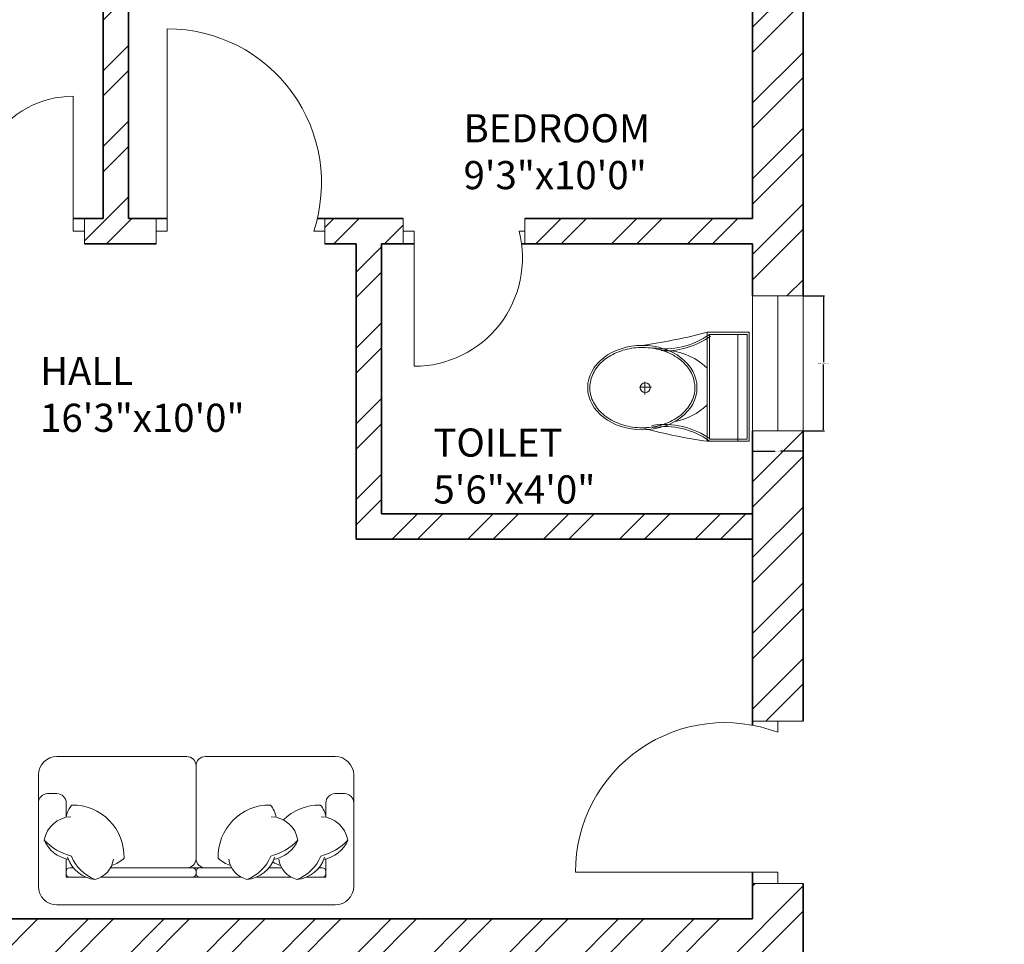
# Model space of a CAD drawing. Units: inches. Extents: x 2552 to 3217, y 1417 to 2737.
# Tile 10 of 25: x 2710 to 2885, y 2138 to 2302. Entities that reach past the tile are written whole.
import ezdxf

# ---------------------------------------------------------------- set-up
doc = ezdxf.new("R2010")
doc.units = ezdxf.units.IN
for name, color, linetype, lineweight in [('A-ANNO-DIMS', 2, 'Continuous', 18), ('A-AREA-IDEN', 7, 'Continuous', 18), ('A-DOOR', 21, 'Continuous', 18), ('A-FLOR-FIXT', 8, 'Continuous', 18), ('A-FURN', 8, 'Continuous', 13), ('A-GLAZ', 161, 'Continuous', 18), ('A-WALL', 7, 'Continuous', 35), ('A-WALL-PATT', 217, 'Continuous', 13)]:
    doc.layers.add(name, color=color, linetype=linetype, lineweight=lineweight)
doc.styles.get("Standard").update_dxf_attribs({"font": 'arial.ttf'})
doc.dimstyles.get("Standard").update_dxf_attribs({"dimtxt": 0.18, "dimasz": 0.18, "dimexe": 0.18, "dimexo": 0.0625, "dimgap": 0.09, "dimtad": 0, "dimtih": 1, "dimtoh": 1, "dimdec": 4, "dimzin": 0, "dimdsep": 46, "dimtxsty": 'Standard', "dimcen": 0.09, "dimadec": 0, "dimazin": 0, "dimtfac": 1, "dimtdec": 4, "dimtofl": 0, "dimtmove": 0, "dimatfit": 3, "dimfxl": 1, "dimtolj": 1, "dimtzin": 0, "dimarcsym": 0})

# ---------------------------------------------------------------- blocks, each defined once
blk = doc.blocks.new('A$C31115884')
for p, q in [((257.5, 466.4), (257.5, 523.2)), ((283.1, 497.7), (223.4, 497.7)), ((0, 200), (0, 0)), ((520, 200), (0, 200)), ((10, 190), (10, 10)), ((510, 190), (10, 190)), ((510, 10), (510, 190)), ((520, 0), (520, 200)), ((510, 54.5), (0, 54.5)), ((10, 10), (510, 10)), ((0, 0), (520, 0))]:
    blk.add_line(p, q)
blk.add_circle((255.6, 496.4), 23.6)
for centre, radius, start, end in [((2777.7, -204.6), 2807, 165.4549, 171.7133), ((3237, 905), 2807, 188.2867, 194.5451), ((-294.5, 403.3), 364.7, 324.2091, 9.3499), ((-294.5, 403.3), 374.7, 324.2091, 9.3499), ((805.8, 403.3), 364.7, 170.6501, 215.7909), ((139.5, 406.2), 293.5, 315.8436, 2.6563), ((805.8, 403.3), 374.7, 179.2036, 215.7909), ((383.6, 406.2), 293.5, 190.2774, 224.1564)]:
    blk.add_arc(centre, radius, start, end)
blk.add_ellipse((256.2, 509.9), major_axis=(0, -260.7), ratio=0.772727)
blk.add_open_spline([(256.2, 259.2), (263.1, 259.2), (270, 259.7), (287.8, 262.3), (298.7, 265.1), (319.9, 273.1), (330.2, 278.4), (350.1, 291.1), (359.7, 298.7), (377.7, 315.9), (386.2, 325.5), (401.7, 346.6), (408.8, 358.1), (421.3, 382.5), (426.8, 395.5), (435.9, 422.4), (439.5, 436.4), (444.8, 465.1), (446.5, 479.7), (447.9, 509.2), (447.6, 524), (445, 553.3), (442.7, 567.8), (436.3, 596), (432.1, 609.7), (421.9, 636), (416, 648.6), (402.5, 672.1), (395, 683), (378.6, 703), (369.8, 712.1), (351.1, 728), (341.3, 734.8), (320.9, 746.2), (310.4, 750.7), (288.9, 757.3), (278, 759.4), (256, 761), (245, 760.6), (223.1, 757.2), (212.3, 754.3), (191.1, 746.1), (180.8, 740.7), (160.9, 727.8), (151.4, 720.1), (133.5, 702.7), (125.1, 693), (109.6, 671.7), (102.6, 660.2), (90.2, 635.7), (84.9, 622.7), (76, 595.6), (72.4, 581.6), (67.2, 552.9), (65.6, 538.2), (64.4, 508.8), (64.8, 494), (67.5, 464.7), (69.9, 450.2), (76.6, 422), (80.8, 408.3), (91.1, 382.2), (97.2, 369.7), (110.8, 346.3), (118.4, 335.4), (134.8, 315.6), (143.7, 306.7), (162.4, 290.9), (172.3, 284.2), (192.8, 273), (203.3, 268.6), (224.8, 262.2), (235.8, 260.2), (249.9, 259.3), (253, 259.2), (256.2, 259.2)], degree=3, knots=[0, 0, 0, 0, 0.110105, 0.110105, 0.285049, 0.285049, 0.459994, 0.459994, 0.634938, 0.634938, 0.809882, 0.809882, 0.984827, 0.984827, 1.159771, 1.159771, 1.334715, 1.334715, 1.50966, 1.50966, 1.684604, 1.684604, 1.859549, 1.859549, 2.034493, 2.034493, 2.209437, 2.209437, 2.384382, 2.384382, 2.559326, 2.559326, 2.73427, 2.73427, 2.909215, 2.909215, 3.084159, 3.084159, 3.259103, 3.259103, 3.434048, 3.434048, 3.608992, 3.608992, 3.783936, 3.783936, 3.958881, 3.958881, 4.133825, 4.133825, 4.30877, 4.30877, 4.483714, 4.483714, 4.658658, 4.658658, 4.833603, 4.833603, 5.008547, 5.008547, 5.183491, 5.183491, 5.358436, 5.358436, 5.53338, 5.53338, 5.708324, 5.708324, 5.883269, 5.883269, 6.058213, 6.058213, 6.233158, 6.233158, 6.283185, 6.283185, 6.283185, 6.283185])
blk = doc.blocks.new('WIN-24')
for p, q in [((0, 24), (9, 24)), ((0, 24), (0, 0)), ((9, 24), (4.5, 24)), ((4.5, 24), (4.5, 0)), ((9, 24), (9, 0)), ((4.5, 0), (0, 0)), ((0, 0), (9, 0))]:
    blk.add_line(p, q)
blk = doc.blocks.new('*D25')
at = {"layer": 'A-ANNO-DIMS', "color": 0, "lineweight": -2, "transparency": 16777216}
for p, q in [((2848.92, 2253.28), (2852.63, 2253.28)), ((2852.45, 2253.1), (2852.45, 2241.47)), ((2852.45, 2229.46), (2852.45, 2241.1)), ((2848.92, 2229.28), (2852.63, 2229.28))]:
    blk.add_line(p, q, dxfattribs=at)
at = {"layer": 'A-ANNO-DIMS', "color": 0, "transparency": 16777216}
for points in [[(2852.42, 2253.1), (2852.48, 2253.1), (2852.45, 2253.28)], [(2852.42, 2229.46), (2852.48, 2229.46), (2852.45, 2229.28)]]:
    blk.add_solid(points, dxfattribs=at)
at = {"layer": 'Defpoints', "color": 0, "transparency": 16777216}
for p in [(2848.85, 2253.28), (2852.45, 2253.28), (2848.85, 2229.28)]:
    blk.add_point(p, dxfattribs=at)
at = {"layer": 'A-ANNO-DIMS', "color": 0, "transparency": 16777216, "insert": (2852.45, 2241.28), "char_height": 0.18, "attachment_point": 5}
blk.add_mtext('\\A1;WINDOW 24 TYP.', dxfattribs=at)
blk = doc.blocks.new('*D26')
at = {"layer": 'A-ANNO-DIMS', "color": 0, "lineweight": -2, "transparency": 16777216}
for p, q in [((2839.85, 2229.22), (2839.85, 2225.5)), ((2848.85, 2229.22), (2848.85, 2225.5)), ((2840.03, 2225.68), (2843.9, 2225.68)), ((2848.67, 2225.68), (2844.81, 2225.68))]:
    blk.add_line(p, q, dxfattribs=at)
at = {"layer": 'A-ANNO-DIMS', "color": 0, "transparency": 16777216}
for points in [[(2840.03, 2225.71), (2840.03, 2225.65), (2839.85, 2225.68)], [(2848.67, 2225.71), (2848.67, 2225.65), (2848.85, 2225.68)]]:
    blk.add_solid(points, dxfattribs=at)
at = {"layer": 'Defpoints', "color": 0, "transparency": 16777216}
for p in [(2839.85, 2229.28), (2848.85, 2229.28), (2848.85, 2225.68)]:
    blk.add_point(p, dxfattribs=at)
at = {"layer": 'A-ANNO-DIMS', "color": 0, "transparency": 16777216, "insert": (2844.35, 2225.68), "char_height": 0.18, "attachment_point": 5}
blk.add_mtext('\\A1;9 TYP.', dxfattribs=at)
blk = doc.blocks.new('*D64')
at = {"layer": 'A-ANNO-DIMS', "color": 0, "lineweight": -2, "transparency": 16777216}
for p, q in [((2646.35, 1551.58), (2646.35, 2709.49)), ((2646.53, 2709.31), (2802.77, 2709.31)), ((2959.93, 2709.31), (2803.69, 2709.31)), ((2960.11, 1551.58), (2960.11, 2709.49))]:
    blk.add_line(p, q, dxfattribs=at)
at = {"layer": 'A-ANNO-DIMS', "color": 0, "transparency": 16777216}
for points in [[(2646.53, 2709.34), (2646.53, 2709.28), (2646.35, 2709.31)], [(2959.93, 2709.34), (2959.93, 2709.28), (2960.11, 2709.31)]]:
    blk.add_solid(points, dxfattribs=at)
at = {"layer": 'Defpoints', "color": 0, "transparency": 16777216}
for p in [(2960.11, 2709.31), (2646.35, 1551.51), (2960.11, 1551.51)]:
    blk.add_point(p, dxfattribs=at)
at = {"layer": 'A-ANNO-DIMS', "color": 0, "transparency": 16777216, "insert": (2803.23, 2709.31), "char_height": 0.18, "attachment_point": 5}
blk.add_mtext('\\A1;313.76', dxfattribs=at)

msp = doc.modelspace()

# ---------------------------------------------------------------- hatches: boundary and pattern name
at = {"layer": 'A-WALL-PATT'}
h = msp.add_hatch(dxfattribs=at)
h.set_pattern_fill('ANSI32', color=256)
h.paths.add_polyline_path([(2756.676, 2649.5125), (2637.3535, 2649.5125), (2637.3535, 2617.9626), (2641.8535, 2617.9626), (2646.3535, 2617.9626), (2646.3535, 2640.5125), (2724.3535, 2640.5125), (2724.3535, 2520.5125), (2720.299, 2520.5125), (2720.299, 2516.0125), (2733.4075, 2516.0125), (2733.4075, 2518.2213), (2733.4075, 2520.5125), (2728.8535, 2520.5125), (2728.8535, 2640.5125), (2756.676, 2640.5125)])
h.paths.add_polyline_path([(2848.8535, 2649.5125), (2804.676, 2649.5125), (2804.676, 2640.5125), (2839.8535, 2640.5125), (2839.8535, 2598.3517), (2848.8535, 2598.3517)])
h.paths.add_polyline_path([(2646.3535, 2516.0125), (2697.9593, 2516.0125), (2697.9593, 2518.2625), (2697.9593, 2520.5125), (2646.3535, 2520.5125), (2646.3535, 2581.9626), (2637.3535, 2581.9626), (2637.3535, 2364.3298), (2646.3535, 2364.3298), (2646.3535, 2387.0125), (2724.3535, 2387.0125), (2724.3535, 2267.0125), (2721.0443, 2267.0125), (2721.0443, 2262.5125), (2733.7854, 2262.5125), (2733.7854, 2264.7625), (2733.7854, 2267.0125), (2728.8535, 2267.0125), (2728.8535, 2387.0125), (2839.8535, 2387.0125), (2839.8535, 2363.8387), (2848.8535, 2363.8387), (2848.8535, 2403.7415), (2844.3535, 2403.7415), (2839.8535, 2403.7415), (2839.8535, 2396.0125), (2646.3535, 2396.0125)])
h.paths.add_polyline_path([(2848.8535, 2550.3517), (2844.3535, 2550.3517), (2839.8535, 2550.3517), (2839.8535, 2520.5125), (2801.9195, 2520.5125), (2801.9195, 2518.2625), (2801.9195, 2516.0125), (2839.8535, 2516.0125), (2839.8535, 2507.5813), (2848.8535, 2507.5813)], flags=17)
h.paths.add_polyline_path([(2848.8535, 2483.5813), (2844.3535, 2483.5813), (2839.8535, 2483.5813), (2839.8535, 2468.0125), (2773.8535, 2468.0125), (2773.8535, 2516.0125), (2778.1336, 2516.0125), (2778.1336, 2520.5125), (2766.696, 2520.5125), (2766.696, 2518.2625), (2766.696, 2516.0125), (2769.3535, 2516.0125), (2769.3535, 2463.5125), (2839.8535, 2463.5125), (2839.8535, 2431.0782), (2848.8535, 2431.0782)], flags=17)
h.paths.add_polyline_path([(2917.8535, 2569.2764), (2913.3535, 2569.2764), (2908.8535, 2569.2764), (2908.8535, 2433.001), (2917.8535, 2433.001), (2917.8535, 2516.0125), (2967.486, 2516.0125), (2967.486, 2520.5125), (2917.8535, 2520.5125)])
h.paths.add_polyline_path([(3000.3535, 2640.5125), (2995.8535, 2640.5125), (2995.8535, 2520.5125), (2990.688, 2520.5125), (2990.688, 2516.0125), (3004.0844, 2516.0125), (3004.0844, 2518.2625), (3004.0844, 2520.5125), (3000.3535, 2520.5125)])
h.paths.add_polyline_path([(3120.3535, 2561.3689), (3115.8535, 2561.3689), (3111.3535, 2561.3689), (3111.3535, 2520.5125), (3070.9814, 2520.5125), (3070.9814, 2518.2625), (3070.9814, 2516.0125), (3111.3535, 2516.0125), (3111.3535, 2505.1841), (3120.3535, 2505.1841)])
h.paths.add_polyline_path([(3120.3535, 2481.1841), (3115.8535, 2481.1841), (3111.3535, 2481.1841), (3111.3535, 2468.0125), (3045.3535, 2468.0125), (3045.3535, 2516.0125), (3048.9787, 2516.0125), (3048.9787, 2520.5125), (3036.3395, 2520.5125), (3036.3395, 2516.0125), (3040.8535, 2516.0125), (3040.8535, 2463.5125), (3111.3535, 2463.5125), (3111.3535, 2396.0125), (2917.8535, 2396.0125), (2917.8535, 2403.4124), (2913.3535, 2403.4124), (2908.8535, 2403.4124), (2908.8535, 2182.5756), (2917.8535, 2182.5756), (2917.8535, 2262.5125), (2968.001, 2262.5125), (2968.001, 2264.7625), (2968.001, 2267.0125), (2917.8535, 2267.0125), (2917.8535, 2387.0125), (3111.3535, 2387.0125), (3111.3535, 2352.2435), (3120.3535, 2352.2435)])
h.paths.add_polyline_path([(3120.3535, 2304.2435), (3115.8535, 2304.2435), (3111.3535, 2304.2435), (3111.3535, 2267.0125), (3073.8616, 2267.0125), (3073.8616, 2264.7625), (3073.8616, 2262.5125), (3111.3535, 2262.5125), (3111.3535, 2252.376), (3120.3535, 2252.376)], flags=17)
h.paths.add_polyline_path([(3120.3535, 2228.376), (3115.8535, 2228.376), (3111.3535, 2228.376), (3111.3535, 2214.5125), (3045.3535, 2214.5125), (3045.3535, 2262.5125), (3049.3096, 2262.5125), (3049.3096, 2267.0125), (3035.0125, 2267.0125), (3035.0125, 2262.5125), (3040.8535, 2262.5125), (3040.8535, 2210.0125), (3111.3535, 2210.0125), (3111.3535, 2142.5125), (2917.8535, 2142.5125), (2917.8535, 2150.2408), (2913.3535, 2150.2408), (2908.8535, 2150.2408), (2908.8535, 1924.9905), (2917.8535, 1924.9905), (2917.8535, 2009.0125), (2971.959, 2009.0125), (2971.959, 2011.2625), (2971.959, 2013.5125), (2917.8535, 2013.5125), (2917.8535, 2133.5125), (2995.8535, 2133.5125), (2995.8535, 2013.5125), (2992.1797, 2013.5125), (2992.1797, 2009.0125), (3004.3344, 2009.0125), (3004.3344, 2011.2625), (3004.3344, 2013.5125), (3000.3535, 2013.5125), (3000.3535, 2133.5125), (3111.3535, 2133.5125), (3111.3535, 2115.0291), (3120.3535, 2115.0291)])
h.paths.add_polyline_path([(3000.3535, 2387.0125), (2995.8535, 2387.0125), (2995.8535, 2267.0125), (2991.3326, 2267.0125), (2991.3326, 2262.5125), (3004.1044, 2262.5125), (3004.1044, 2264.7625), (3004.1044, 2267.0125), (3000.3535, 2267.0125)], flags=17)
h.paths.add_polyline_path([(3120.3535, 1973.2388), (3115.8535, 1973.2388), (3111.3535, 1973.2388), (3111.3535, 1961.0125), (3045.3535, 1961.0125), (3045.3535, 2009.0125), (3048.9101, 2009.0125), (3048.9101, 2013.5125), (3037.105, 2013.5125), (3037.105, 2011.2625), (3037.105, 2009.0125), (3040.8535, 2009.0125), (3040.8535, 1956.5125), (3111.3535, 1956.5125), (3111.3535, 1889.0125), (2917.8535, 1889.0125), (2917.8535, 1895.7215), (2913.3535, 1895.7215), (2908.8535, 1895.7215), (2908.8535, 1844.2217), (2917.8535, 1844.2217), (2917.8535, 1880.0125), (3111.3535, 1880.0125), (3111.3535, 1846.9541), (3120.3535, 1846.9541)])
h.paths.add_polyline_path([(3120.3535, 2067.0291), (3111.3535, 2067.0291), (3111.3535, 2013.5125), (3071.3001, 2013.5125), (3071.3001, 2009.0125), (3111.3535, 2009.0125), (3111.3535, 1997.2388), (3120.3535, 1997.2388)], flags=0)
h.paths.add_polyline_path([(3120.3535, 1798.9541), (3115.8535, 1798.9541), (3111.3535, 1798.9541), (3111.3535, 1760.0125), (3071.2497, 1760.0125), (3071.2497, 1757.7625), (3071.2497, 1755.5125), (3111.3535, 1755.5125), (3111.3535, 1746.162), (3120.3535, 1746.2478)])
h.paths.add_polyline_path([(3120.3535, 1722.2049), (3111.3535, 1722.2049), (3111.3535, 1707.5125), (3045.3535, 1707.5125), (3045.3535, 1755.5125), (3048.6624, 1755.5125), (3048.6624, 1760.0125), (3035.3703, 1760.0125), (3035.3703, 1755.5125), (3040.8535, 1755.5125), (3040.8535, 1703.0125), (3111.3535, 1703.0125), (3111.3535, 1635.5125), (2917.8535, 1635.5125), (2917.8535, 1643.1366), (2913.3535, 1643.1366), (2908.8535, 1643.1366), (2908.8535, 1626.5125), (3120.3535, 1626.5125)])
h.paths.add_polyline_path([(2917.8535, 1755.5125), (2973.2287, 1755.5125), (2973.2287, 1757.7625), (2973.2287, 1760.0125), (2917.8535, 1760.0125), (2917.8535, 1808.2217), (2913.3535, 1808.2217), (2908.8535, 1808.2217), (2908.8535, 1676.1665), (2917.8535, 1676.1665)])
h.paths.add_polyline_path([(3000.3535, 1880.0125), (2995.8535, 1880.0125), (2995.8535, 1760.0125), (2992.9329, 1760.0125), (2992.9329, 1755.5125), (3003.8766, 1755.5125), (3003.8766, 1757.7625), (3003.8766, 1760.0125), (3000.3535, 1760.0125)])
h.paths.add_polyline_path([(2848.8535, 1896.6971), (2844.3535, 1896.6971), (2839.8535, 1896.6971), (2839.8535, 1889.0125), (2646.3535, 1889.0125), (2646.3535, 2009.0125), (2700.5253, 2009.0125), (2700.5253, 2011.2625), (2700.5253, 2013.5125), (2646.3535, 2013.5125), (2646.3535, 2053.1812), (2641.8535, 2053.1812), (2637.3535, 2053.1812), (2637.3535, 1836.254), (2646.3535, 1836.254), (2646.3535, 1880.0125), (2724.3535, 1880.0125), (2724.3535, 1760.0125), (2721.2473, 1760.0125), (2721.2473, 1755.5125), (2731.9187, 1755.5125), (2731.9187, 1757.7625), (2731.9187, 1760.0125), (2728.8535, 1760.0125), (2728.8535, 1880.0125), (2839.8535, 1880.0125), (2839.8535, 1840.3813), (2848.8535, 1840.3813)])
h.paths.add_polyline_path([(2848.8535, 1792.3813), (2844.3535, 1792.3813), (2839.8535, 1792.3813), (2839.8535, 1760.0125), (2797.8845, 1760.0125), (2797.8845, 1755.5125), (2839.8535, 1755.5125), (2839.8535, 1743.3688), (2844.3535, 1743.3688), (2848.8535, 1743.3688)], flags=0)
h.paths.add_polyline_path([(2848.8535, 1719.3688), (2844.3535, 1719.3688), (2839.8535, 1719.3688), (2839.8535, 1707.5125), (2773.8535, 1707.5125), (2773.8535, 1755.5125), (2777.716, 1755.5125), (2777.716, 1760.0125), (2760.9247, 1760.0125), (2760.9247, 1757.9721), (2760.9247, 1755.5125), (2769.3535, 1755.5125), (2769.3535, 1703.0125), (2839.8535, 1703.0125), (2839.8535, 1673.0277), (2848.8535, 1672.9407)], flags=0)
h.paths.add_polyline_path([(2646.3535, 1755.5125), (2702.9171, 1755.5125), (2702.9171, 1757.7625), (2702.9171, 1760.0125), (2646.3535, 1760.0125), (2646.3535, 1800.254), (2641.8535, 1800.254), (2637.3535, 1800.254), (2637.3535, 1626.5125), (2848.8535, 1626.5125), (2848.8535, 1643.1187), (2844.3535, 1643.1187), (2839.8535, 1643.1187), (2839.8535, 1635.5125), (2646.3535, 1635.5125)])
h.paths.add_polyline_path([(2848.8535, 2148.8427), (2844.3535, 2148.8427), (2839.8535, 2148.8427), (2839.8535, 2142.5125), (2646.3535, 2142.5125), (2646.3535, 2262.5125), (2701.3562, 2262.5125), (2701.3562, 2264.7625), (2701.3562, 2267.0125), (2646.3535, 2267.0125), (2646.3535, 2328.3298), (2637.3535, 2328.3298), (2637.3535, 2089.1812), (2646.3535, 2089.1812), (2646.3535, 2133.5125), (2839.8535, 2133.5125), (2839.8535, 2097.5966), (2848.8535, 2097.5966)])
h.paths.add_polyline_path([(2728.8535, 2133.5125), (2724.3535, 2133.5125), (2724.3535, 2013.5125), (2719.6039, 2013.5125), (2719.6039, 2009.0125), (2732.5784, 2009.0125), (2732.5784, 2011.2625), (2732.5784, 2013.5125), (2728.8535, 2013.5125)])
h.paths.add_polyline_path([(2848.8535, 1970.0557), (2844.3535, 1970.0557), (2839.8535, 1970.0557), (2839.8535, 1961.0125), (2773.8535, 1961.0125), (2773.8535, 2009.0125), (2777.3388, 2009.0125), (2777.3388, 2013.5125), (2764.7681, 2013.5125), (2764.7681, 2009.0125), (2769.3535, 2009.0125), (2769.3535, 1956.5125), (2839.8535, 1956.5125), (2839.8535, 1924.7199), (2848.8535, 1924.7199)], flags=17)
h.paths.add_polyline_path([(2848.8535, 2049.5966), (2844.3535, 2049.5966), (2839.8535, 2049.5966), (2839.8535, 2013.5125), (2798.198, 2013.5125), (2798.198, 2011.2625), (2798.198, 2009.0125), (2839.8535, 2009.0125), (2839.8535, 1994.0557), (2848.8535, 1994.0557)], flags=17)
h.paths.add_polyline_path([(2848.8535, 2315.8387), (2839.8535, 2315.8387), (2839.8535, 2267.0125), (2799.3375, 2267.0125), (2799.3375, 2264.7625), (2799.3375, 2262.5125), (2839.8535, 2262.5125), (2839.8535, 2253.2843), (2848.8535, 2253.2843)], flags=17)
h.paths.add_polyline_path([(2848.8535, 2229.2843), (2839.8535, 2229.2843), (2839.8535, 2177.6936), (2848.8535, 2177.6936)], flags=17)
h.paths.add_polyline_path([(2839.8535, 2214.5125), (2773.8535, 2214.5125), (2773.8535, 2262.5125), (2777.6984, 2262.5125), (2777.6984, 2267.0125), (2763.8226, 2267.0125), (2763.8226, 2262.5125), (2769.3535, 2262.5125), (2769.3535, 2210.0125), (2839.8535, 2210.0125)], flags=17)
h.paths.add_polyline_path([(3050.32, 2520.2817), (3088.9114, 2520.2817), (3088.9114, 2538.939), (3050.32, 2538.939)], flags=9)

# ---------------------------------------------------------------- linework, layer by layer
at = {"layer": 'A-DOOR'}
for p, q in [((2735.7854, 2264.7625), (2735.7854, 2300.7625)), ((2719.0443, 2264.7625), (2719.0443, 2288.7625)), ((2721.0443, 2267.0125), (2721.0443, 2262.5125)), ((2733.7854, 2267.0125), (2733.7854, 2262.5125)), ((2763.8226, 2267.0125), (2763.8226, 2262.5125)), ((2777.6984, 2262.5125), (2777.6984, 2267.0125)), ((2777.6984, 2267.0125), (2777.6984, 2264.7625)), ((2799.3375, 2262.5125), (2799.3375, 2267.0125)), ((2799.3375, 2267.0125), (2799.3375, 2264.7625)), ((2721.0443, 2264.7625), (2719.0443, 2264.7625)), ((2721.0443, 2262.5125), (2721.0443, 2264.7625)), ((2733.7854, 2262.5125), (2733.7854, 2264.7625)), ((2733.7854, 2264.7625), (2735.7854, 2264.7625)), ((2763.8226, 2264.7625), (2761.8226, 2264.7625)), ((2763.8226, 2262.5125), (2763.8226, 2264.7625)), ((2777.6984, 2264.7625), (2779.6984, 2264.7625)), ((2779.6984, 2264.7625), (2779.6984, 2240.7625)), ((2799.3375, 2264.7625), (2798.3375, 2264.7625)), ((2839.8535, 2177.6936), (2848.8535, 2177.6936)), ((2848.8535, 2177.6936), (2844.3535, 2177.6936)), ((2844.3535, 2177.6936), (2844.3535, 2175.6936)), ((2844.3535, 2150.8427), (2808.3535, 2150.8427)), ((2844.3535, 2148.8427), (2844.3535, 2150.8427)), ((2839.8535, 2148.8427), (2848.8535, 2148.8427)), ((2848.8535, 2148.8427), (2844.3535, 2148.8427))]:
    msp.add_line(p, q, dxfattribs=at)
for centre, radius, start, end in [((2735.7854, 2273.3467), 27.4158, 341.753227, 90), ((2719.0443, 2271.6351), 17.1274, 90, 203.657264), ((2779.6984, 2260.0003), 19.2378, 270, 14.332344), ((2834.9308, 2150.8427), 26.5773, 69.23481, 180)]:
    msp.add_arc(centre, radius, start, end, dxfattribs=at)
at = {"layer": 'A-FURN', "ltscale": 0.03}
msp.add_lwpolyline([(2739.2443, 2171.3947, -0.41421356), (2740.8938, 2169.7451, -0.41421356), (2742.5434, 2171.3947), (2765.6373, 2171.3947, -0.41421356), (2768.9364, 2168.0956), (2768.9364, 2148.3008, -0.41421356), (2765.6373, 2145.0017), (2716.1504, 2145.0017, -0.41421356), (2712.8513, 2148.3008), (2712.8513, 2168.0956, -0.41421356), (2716.1504, 2171.3947), (2739.2443, 2171.3947, -0.41421356), (2740.8938, 2169.7451, -0.41421356), (2742.5434, 2171.3947)], format="xyb", dxfattribs=at)
msp.add_lwpolyline([(2739.2443, 2171.3947, -0.41421356), (2740.8938, 2169.7451, -0.41421356), (2742.5434, 2171.3947), (2765.6373, 2171.3947, -0.41421356), (2768.9364, 2168.0956), (2768.9364, 2148.3008, -0.41421356), (2765.6373, 2145.0017), (2716.1504, 2145.0017, -0.41421356), (2712.8513, 2148.3008), (2712.8513, 2168.0956, -0.41421356), (2716.1504, 2171.3947), (2739.2443, 2171.3947, -0.41421356), (2740.8938, 2169.7451, -0.41421356), (2742.5434, 2171.3947)], format="xyb", dxfattribs=at)
at = {"layer": 'A-FURN'}
for points in [[(2739.2443, 2151.5999, 0.41421356), (2740.8938, 2153.2495), (2740.8938, 2169.7451, 0.41421356)], [(2739.2443, 2151.5999, 0.41421356), (2740.8938, 2153.2495), (2740.8938, 2169.7451, 0.41421356)], [(2742.5434, 2151.5999, -0.41421356), (2740.8938, 2153.2495), (2740.8938, 2169.7451, -0.41421356)], [(2742.5434, 2151.5999, -0.41421356), (2740.8938, 2153.2495), (2740.8938, 2169.7451, -0.41421356)], [(2712.8513, 2163.1469, -0.41421356), (2714.5008, 2164.7965), (2716.1504, 2164.7965, -0.41421356), (2717.8, 2163.1469), (2717.8, 2160.5911)], [(2712.8513, 2163.1469, -0.41421356), (2714.5008, 2164.7965), (2716.1504, 2164.7965, -0.41421356), (2717.8, 2163.1469), (2717.8, 2160.5911)], [(2763.9877, 2160.5911), (2763.9877, 2163.1469, -0.41421356), (2765.6373, 2164.7965), (2767.2869, 2164.7965, -0.41421356), (2768.9364, 2163.1469)], [(2763.9877, 2160.5911), (2763.9877, 2163.1469, -0.41421356), (2765.6373, 2164.7965), (2767.2869, 2164.7965, -0.41421356), (2768.9364, 2163.1469)], [(2717.7964, 2160.5904, -0.16554063), (2718.8168, 2162.7699, -0.42598917), (2728.0811, 2153.3201, -0.12152332), (2725.8819, 2152.0176, 7.11546429)], [(2717.7964, 2160.5904, -0.16554063), (2718.8168, 2162.7699, -0.42598917), (2728.0811, 2153.3201, -0.12152332), (2725.8819, 2152.0176, 7.11546429)], [(2755.1052, 2160.5904, 0.16554063), (2754.0847, 2162.7699, 0.42598917), (2744.8204, 2153.3201, 0.12152332), (2747.0196, 2152.0176, -7.11546429)], [(2755.1052, 2160.5904, 0.16554063), (2754.0847, 2162.7699, 0.42598917), (2744.8204, 2153.3201, 0.12152332), (2747.0196, 2152.0176, -7.11546429)], [(2763.9913, 2160.5904, 0.16554063), (2762.9708, 2162.7699, 0.20023115), (2756.4227, 2160.1154, 0.12152332)], [(2763.9913, 2160.5904, 0.16554063), (2762.9708, 2162.7699, 0.20023115), (2756.4227, 2160.1154, 0.12152332)], [(2718.6278, 2160.6909, 0.35677236), (2713.9011, 2156.533, 0.24954205), (2718.1839, 2153.1066, -9.61688035)], [(2718.6278, 2160.6909, 0.35677236), (2713.9011, 2156.533, 0.24954205), (2718.1839, 2153.1066, -9.61688035)], [(2754.2738, 2160.6909, -0.35677236), (2759.0004, 2156.533, -0.24954205), (2754.7177, 2153.1066, 9.61688035)], [(2754.2738, 2160.6909, -0.35677236), (2759.0004, 2156.533, -0.24954205), (2754.7177, 2153.1066, 9.61688035)], [(2763.1599, 2160.6909, -0.35677236), (2767.8866, 2156.533, -0.24954205), (2763.6038, 2153.1066, 9.61688035)], [(2763.1599, 2160.6909, -0.35677236), (2767.8866, 2156.533, -0.24954205), (2763.6038, 2153.1066, 9.61688035)], [(2713.9011, 2156.533, 0.14772988), (2718.7223, 2153.6981, 0.21334276), (2722.9763, 2149.5402, 0.17866181)], [(2713.9011, 2156.533, 0.14772988), (2718.7223, 2153.6981, 0.21334276), (2722.9763, 2149.5402, 0.17866181)], [(2759.0004, 2156.533, -0.14772988), (2754.1792, 2153.6981, -0.21334276), (2749.9252, 2149.5402, -0.17866181)], [(2759.0004, 2156.533, -0.14772988), (2754.1792, 2153.6981, -0.21334276), (2749.9252, 2149.5402, -0.17866181)], [(2767.8866, 2156.533, -0.14772988), (2763.0654, 2153.6981, -0.21334276), (2758.8114, 2149.5402, -0.17866181)], [(2767.8866, 2156.533, -0.14772988), (2763.0654, 2153.6981, -0.21334276), (2758.8114, 2149.5402, -0.17866181)], [(2718.0563, 2153.4722, 0.30666349), (2722.9763, 2149.5402, 0.30632997), (2726.1904, 2153.1311, -0.87284716)], [(2718.0563, 2153.4722, 0.30666349), (2722.9763, 2149.5402, 0.30632997), (2726.1904, 2153.1311, -0.87284716)], [(2739.2443, 2151.5999, 0.41421356), (2740.8938, 2153.2495)], [(2739.2443, 2151.5999, 0.41421356), (2740.8938, 2153.2495)], [(2742.5434, 2151.5999, -0.41421356), (2740.8938, 2153.2495)], [(2742.5434, 2151.5999, -0.41421356), (2740.8938, 2153.2495)], [(2754.8453, 2153.4722, -0.30666349), (2749.9252, 2149.5402, -0.30632997), (2746.7111, 2153.1311, 0.87284716)], [(2754.8453, 2153.4722, -0.30666349), (2749.9252, 2149.5402, -0.30632997), (2746.7111, 2153.1311, 0.87284716)], [(2754.5228, 2152.6625, 0.07186538), (2755.9057, 2152.0176, -7.11546429)], [(2754.5228, 2152.6625, 0.07186538), (2755.9057, 2152.0176, -7.11546429)], [(2763.7314, 2153.4722, -0.30666349), (2758.8114, 2149.5402, -0.30632997), (2755.5972, 2153.1311, 0.87284716)], [(2763.7314, 2153.4722, -0.30666349), (2758.8114, 2149.5402, -0.30632997), (2755.5972, 2153.1311, 0.87284716)], [(2760.5175, 2149.9504), (2763.9877, 2149.9504), (2763.9877, 2153.1922, -0.41421356)], [(2760.5175, 2149.9504), (2763.9877, 2149.9504), (2763.9877, 2153.1922, -0.41421356)], [(2719.0588, 2151.5999), (2718.4598, 2151.5999, 0.41421356), (2717.8, 2150.9401), (2717.8, 2150.6102, 0.41421356), (2718.4598, 2149.9504)], [(2719.0588, 2151.5999), (2718.4598, 2151.5999, 0.41421356), (2717.8, 2150.9401), (2717.8, 2150.6102, 0.41421356), (2718.4598, 2149.9504)], [(2724.0145, 2149.9504), (2740.234, 2149.9504, 0.41421356), (2740.8938, 2150.6102), (2740.8938, 2150.9401, 0.41421356), (2740.234, 2151.5999), (2725.6755, 2151.5999, 0.41421356)], [(2724.0145, 2149.9504), (2740.234, 2149.9504, 0.41421356), (2740.8938, 2150.6102), (2740.8938, 2150.9401, 0.41421356), (2740.234, 2151.5999), (2725.6755, 2151.5999, 0.41421356)], [(2748.8871, 2149.9504), (2741.5537, 2149.9504, -0.41421356), (2740.8938, 2150.6102), (2740.8938, 2150.9401, -0.41421356), (2741.5537, 2151.5999), (2747.2261, 2151.5999, -0.41421356)], [(2748.8871, 2149.9504), (2741.5537, 2149.9504, -0.41421356), (2740.8938, 2150.6102), (2740.8938, 2150.9401, -0.41421356), (2741.5537, 2151.5999), (2747.2261, 2151.5999, -0.41421356)], [(2753.8428, 2151.5999), (2756.1122, 2151.5999, -0.41421356)], [(2753.8428, 2151.5999), (2756.1122, 2151.5999, -0.41421356)], [(2762.7289, 2151.5999), (2763.3279, 2151.5999, -0.41421356), (2763.9877, 2150.9401), (2763.9877, 2150.6102, -0.41421356), (2763.3279, 2149.9504)], [(2762.7289, 2151.5999), (2763.3279, 2151.5999, -0.41421356), (2763.9877, 2150.9401), (2763.9877, 2150.6102, -0.41421356), (2763.3279, 2149.9504)], [(2718.4598, 2149.9504), (2721.2702, 2149.9504, 0.41421356)], [(2718.4598, 2149.9504), (2721.2702, 2149.9504, 0.41421356)], [(2757.7732, 2149.9504), (2751.6314, 2149.9504, -0.41421356)], [(2757.7732, 2149.9504), (2751.6314, 2149.9504, -0.41421356)], [(2763.3279, 2149.9504), (2760.5175, 2149.9504, -0.41421356)], [(2763.3279, 2149.9504), (2760.5175, 2149.9504, -0.41421356)]]:
    msp.add_lwpolyline(points, format="xyb", dxfattribs=at)
for points in [[(2717.8, 2153.1922), (2717.8, 2149.9504), (2721.2702, 2149.9504)], [(2717.8, 2153.1922), (2717.8, 2149.9504), (2721.2702, 2149.9504)], [(2724.0145, 2149.9504), (2748.8871, 2149.9504)], [(2724.0145, 2149.9504), (2748.8871, 2149.9504)], [(2751.6314, 2149.9504), (2757.7732, 2149.9504)], [(2751.6314, 2149.9504), (2757.7732, 2149.9504)]]:
    msp.add_lwpolyline(points, dxfattribs=at)
msp.add_lwpolyline([(2740.234, 2149.9504), (2741.5537, 2149.9504, -0.41421356), (2740.8938, 2150.6102), (2740.8938, 2150.9401, -0.41421356), (2741.5537, 2151.5999), (2740.234, 2151.5999, -0.41421356), (2740.8938, 2150.9401), (2740.8938, 2150.6102, -0.41421356)], format="xyb", close=True, dxfattribs=at)
msp.add_lwpolyline([(2740.234, 2149.9504), (2741.5537, 2149.9504, -0.41421356), (2740.8938, 2150.6102), (2740.8938, 2150.9401, -0.41421356), (2741.5537, 2151.5999), (2740.234, 2151.5999, -0.41421356), (2740.8938, 2150.9401), (2740.8938, 2150.6102, -0.41421356)], format="xyb", close=True, dxfattribs=at)
at = {"layer": 'A-GLAZ'}
for p, q in [((2844.3535, 2253.2843), (2844.3535, 2253.2843)), ((2839.8535, 2229.2843), (2839.8535, 2229.2843))]:
    msp.add_line(p, q, dxfattribs=at)
at = {"layer": 'A-WALL'}
for p, q in [((2724.3535, 2387.0125), (2724.3535, 2267.0125)), ((2728.8535, 2387.0125), (2728.8535, 2267.0125)), ((2839.8535, 2315.8387), (2839.8535, 2267.0125)), ((2848.8535, 2315.8387), (2848.8535, 2253.2843)), ((2719.0443, 2267.0125), (2724.3535, 2267.0125)), ((2728.8535, 2267.0125), (2735.7854, 2267.0125)), ((2762.4594, 2267.0125), (2777.6984, 2267.0125)), ((2799.3375, 2267.0125), (2839.8535, 2267.0125)), ((2721.0443, 2262.5125), (2733.7854, 2262.5125)), ((2763.8226, 2262.5125), (2769.3535, 2262.5125)), ((2769.3535, 2262.5125), (2769.3535, 2210.0125)), ((2773.8535, 2262.5125), (2773.8535, 2214.5125)), ((2773.8535, 2262.5125), (2779.6984, 2262.5125)), ((2798.7715, 2262.5125), (2839.8535, 2262.5125)), ((2839.8535, 2262.5125), (2839.8535, 2253.2843)), ((2839.8535, 2229.2843), (2839.8535, 2176.9602)), ((2848.8535, 2229.2843), (2848.8535, 2177.6936)), ((2773.8535, 2214.5125), (2839.8535, 2214.5125)), ((2769.3535, 2210.0125), (2839.8535, 2210.0125)), ((2839.8535, 2150.8427), (2839.8535, 2142.5125)), ((2848.8535, 2148.8427), (2848.8535, 2097.5966)), ((2646.3535, 2142.5125), (2839.8535, 2142.5125))]:
    msp.add_line(p, q, dxfattribs=at)

# ---------------------------------------------------------------- block references
at = {"layer": 'A-FLOR-FIXT', "xscale": 0.0372717239612423, "yscale": 0.0372717239612423, "zscale": 0.0372717239612423, "rotation": 89.99999999999999}
msp.add_blockref('A$C31115884', (2839.2663, 2227.4243), dxfattribs=at)
at = {"layer": 'A-GLAZ'}
msp.add_blockref('WIN-24', (2839.854, 2229.284), dxfattribs=at)

# ---------------------------------------------------------------- texts
at = {"layer": 'A-AREA-IDEN', "char_height": 5, "attachment_point": 1}
for s, width, insert in [('BEDROOM\\P9\'3"x10\'0"', 103.95052, (2788.4656, 2285.5742)), ('HALL\\P16\'3"x10\'0"', 136.201362, (2713.1618, 2242.4409)), ('TOILET\\P5\'6"x4\'0"', 66.803516, (2783.1083, 2229.6981))]:
    msp.add_mtext_dynamic_manual_height_columns(s, width=width, gutter_width=12.5, heights=[0], dxfattribs=dict(at, insert=insert))

# ---------------------------------------------------------------- dimensions: what is measured, and where the dimension line sits
at = {"layer": 'A-ANNO-DIMS'}
dim = msp.add_linear_dim(base=(2960.1089, 2709.3125), p1=(2646.3535, 1551.5125), p2=(2960.1089, 1551.5125), dimstyle='Standard', override={"dimdec": 2, "dimlfac": 1, "dimrnd": 0, "dimzin": 0, "dimdsep": 46, "dimlunit": 2}, dxfattribs=at)
dim.commit()
dim.dimension.update_dxf_attribs({"geometry": '*D64', "text_midpoint": (2803.2312, 2709.3125)})
dim = msp.add_linear_dim(base=(2852.4535, 2253.2843), p1=(2848.8535, 2229.2843), p2=(2848.8535, 2253.2843), angle=90, text='WINDOW <> TYP.', dimstyle='Standard', override={"dimdec": 0, "dimlfac": 1, "dimrnd": 0, "dimzin": 0, "dimdsep": 46, "dimlunit": 2}, dxfattribs=at)
dim.commit()
dim.dimension.update_dxf_attribs({"geometry": '*D25', "text_midpoint": (2852.4535, 2241.2843)})
dim = msp.add_linear_dim(base=(2848.8535, 2225.6843), p1=(2839.8535, 2229.2843), p2=(2848.8535, 2229.2843), text='<> TYP.', dimstyle='Standard', override={"dimdec": 0, "dimlfac": 1, "dimrnd": 0, "dimzin": 0, "dimdsep": 46, "dimlunit": 2}, dxfattribs=at)
dim.commit()
dim.dimension.update_dxf_attribs({"geometry": '*D26', "text_midpoint": (2844.3535, 2225.6843)})

doc.saveas('drawing.dxf')
